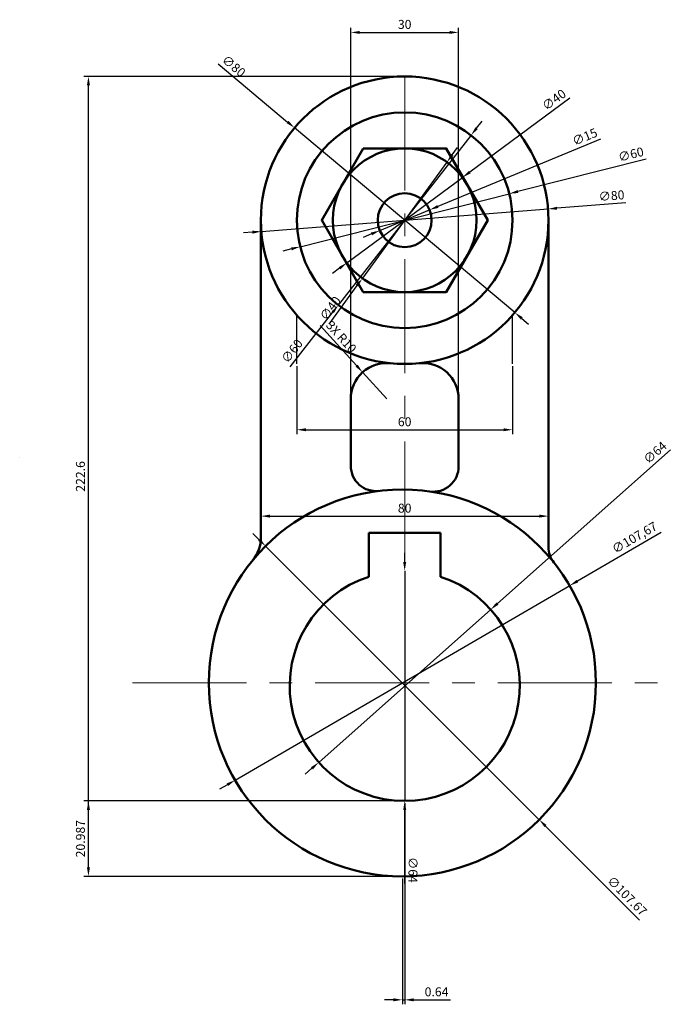
# Model space of a CAD drawing. Units: millimetres. Extents: x 3628 to 3809, y 2625 to 2899.
import ezdxf

# ---------------------------------------------------------------- set-up
doc = ezdxf.new("R2010")
doc.units = ezdxf.units.MM
doc.linetypes.add('CENTER', pattern=[50.8, 31.75, -6.35, 6.35, -6.35])
for name, color, linetype, lineweight in [('M-CNTR', 4, 'CENTER', 18), ('M-CONS', 8, 'Continuous', 13), ('M-DIMS', 2, 'Continuous', 25), ('M-OUTL', 7, 'Continuous', 50)]:
    doc.layers.add(name, color=color, linetype=linetype, lineweight=lineweight)
doc.styles.get("Standard").update_dxf_attribs({"font": 'arial.ttf'})
doc.dimstyles.new('ISO-25', dxfattribs={"dimtxt": 2.5, "dimasz": 2.5, "dimexe": 1.25, "dimexo": 0.625, "dimtad": 1, "dimtxsty": 'Standard', "dimcen": 2.5, "dimadec": 0, "dimazin": 0, "dimtfac": 1, "dimtmove": 0, "dimatfit": 3, "dimfxl": 1, "dimarcsym": 0})

# ---------------------------------------------------------------- blocks, each defined once
blk = doc.blocks.new('*D1')
at = {"layer": 'Defpoints', "color": 0, "transparency": 16777216}
for p in [(3758.59, 2734.73), (3710.75, 2692.22)]:
    blk.add_point(p, dxfattribs=at)
at = {"layer": 'M-DIMS', "color": 0, "lineweight": -2, "transparency": 16777216}
for p, q in [((3808.64, 2779.22), (3760.46, 2736.39)), ((3710.75, 2692.22), (3758.59, 2734.73)), ((3708.88, 2690.56), (3707.02, 2688.9))]:
    blk.add_line(p, q, dxfattribs=at)
at = {"layer": 'M-DIMS', "color": 0, "transparency": 16777216}
for points in [[(3760.18, 2736.71), (3760.74, 2736.08), (3758.59, 2734.73)], [(3708.61, 2690.87), (3709.16, 2690.25), (3710.75, 2692.22)]]:
    blk.add_solid(points, dxfattribs=at)
at = {"layer": 'M-DIMS', "color": 0, "transparency": 16777216, "insert": (3804.52, 2778.19), "char_height": 2.5, "attachment_point": 5, "rotation": 41.628}
blk.add_mtext('∅64', dxfattribs=at)
blk = doc.blocks.new('*D2')
at = {"layer": 'Defpoints', "color": 0, "transparency": 16777216}
for p in [(3750.76, 2854.98), (3718.59, 2831.21)]:
    blk.add_point(p, dxfattribs=at)
at = {"layer": 'M-DIMS', "color": 0, "lineweight": -2, "transparency": 16777216}
for p, q in [((3780.59, 2877.02), (3752.77, 2856.46)), ((3718.59, 2831.21), (3750.76, 2854.98)), ((3716.57, 2829.73), (3714.56, 2828.24))]:
    blk.add_line(p, q, dxfattribs=at)
at = {"layer": 'M-DIMS', "color": 0, "transparency": 16777216}
for points in [[(3752.52, 2856.8), (3753.02, 2856.13), (3750.76, 2854.98)], [(3716.33, 2830.06), (3716.82, 2829.39), (3718.59, 2831.21)]]:
    blk.add_solid(points, dxfattribs=at)
at = {"layer": 'M-DIMS', "color": 0, "transparency": 16777216, "insert": (3776.39, 2876.36), "char_height": 2.5, "attachment_point": 5, "rotation": 36.4548}
blk.add_mtext('∅40', dxfattribs=at)
blk = doc.blocks.new('*D3')
at = {"layer": 'Defpoints', "color": 0, "transparency": 16777216}
for p in [(3741.6, 2845.96), (3727.74, 2840.23)]:
    blk.add_point(p, dxfattribs=at)
at = {"layer": 'M-DIMS', "color": 0, "lineweight": -2, "transparency": 16777216}
for p, q in [((3789.15, 2865.64), (3743.91, 2846.92)), ((3727.74, 2840.23), (3741.6, 2845.96)), ((3725.43, 2839.27), (3723.12, 2838.32))]:
    blk.add_line(p, q, dxfattribs=at)
at = {"layer": 'M-DIMS', "color": 0, "transparency": 16777216}
for points in [[(3743.75, 2847.3), (3744.07, 2846.53), (3741.6, 2845.96)], [(3725.27, 2839.66), (3725.59, 2838.89), (3727.74, 2840.23)]]:
    blk.add_solid(points, dxfattribs=at)
at = {"layer": 'M-DIMS', "color": 0, "transparency": 16777216, "insert": (3784.89, 2866.01), "char_height": 2.5, "attachment_point": 5, "rotation": 22.4807}
blk.add_mtext('∅15', dxfattribs=at)
blk = doc.blocks.new('*D4')
at = {"layer": 'Defpoints', "color": 0, "transparency": 16777216}
for p in [(3763.75, 2850.46), (3705.59, 2835.73)]:
    blk.add_point(p, dxfattribs=at)
at = {"layer": 'M-DIMS', "color": 0, "lineweight": -2, "transparency": 16777216}
for p, q in [((3801.82, 2860.11), (3766.18, 2851.08)), ((3705.59, 2835.73), (3763.75, 2850.46)), ((3703.17, 2835.11), (3700.74, 2834.5))]:
    blk.add_line(p, q, dxfattribs=at)
at = {"layer": 'M-DIMS', "color": 0, "transparency": 16777216}
for points in [[(3766.07, 2851.48), (3766.28, 2850.67), (3763.75, 2850.46)], [(3703.07, 2835.52), (3703.27, 2834.71), (3705.59, 2835.73)]]:
    blk.add_solid(points, dxfattribs=at)
at = {"layer": 'M-DIMS', "color": 0, "transparency": 16777216, "insert": (3797.68, 2861.1), "char_height": 2.5, "attachment_point": 5, "rotation": 14.2196}
blk.add_mtext('∅60', dxfattribs=at)
blk = doc.blocks.new('*D5')
at = {"layer": 'Defpoints', "color": 0, "transparency": 16777216}
for p in [(3774.55, 2846.23), (3694.79, 2839.96)]:
    blk.add_point(p, dxfattribs=at)
at = {"layer": 'M-DIMS', "color": 0, "lineweight": -2, "transparency": 16777216}
for p, q in [((3796.15, 2847.93), (3777.04, 2846.43)), ((3694.79, 2839.96), (3774.55, 2846.23)), ((3692.3, 2839.76), (3689.81, 2839.57))]:
    blk.add_line(p, q, dxfattribs=at)
at = {"layer": 'M-DIMS', "color": 0, "transparency": 16777216}
for points in [[(3777.01, 2846.84), (3777.07, 2846.01), (3774.55, 2846.23)], [(3692.27, 2840.18), (3692.34, 2839.35), (3694.79, 2839.96)]]:
    blk.add_solid(points, dxfattribs=at)
at = {"layer": 'M-DIMS', "color": 0, "transparency": 16777216, "insert": (3792.23, 2849.6), "char_height": 2.5, "attachment_point": 5, "rotation": 4.4985}
blk.add_mtext('∅80', dxfattribs=at)
blk = doc.blocks.new('*D6')
at = {"layer": 'Defpoints', "color": 0, "transparency": 16777216}
for p in [(3704.67, 2803.1), (3764.67, 2803.1), (3764.67, 2784.78)]:
    blk.add_point(p, dxfattribs=at)
at = {"layer": 'M-DIMS', "color": 0, "lineweight": -2, "transparency": 16777216}
for p, q in [((3704.67, 2802.47), (3704.67, 2783.53)), ((3764.67, 2802.47), (3764.67, 2783.53)), ((3707.17, 2784.78), (3762.17, 2784.78))]:
    blk.add_line(p, q, dxfattribs=at)
at = {"layer": 'M-DIMS', "color": 0, "transparency": 16777216}
for points in [[(3707.17, 2785.2), (3707.17, 2784.36), (3704.67, 2784.78)], [(3762.17, 2785.2), (3762.17, 2784.36), (3764.67, 2784.78)]]:
    blk.add_solid(points, dxfattribs=at)
at = {"layer": 'M-DIMS', "color": 0, "transparency": 16777216, "insert": (3734.67, 2786.68), "char_height": 2.5, "attachment_point": 5}
blk.add_mtext('60', dxfattribs=at)
blk = doc.blocks.new('*D7')
at = {"layer": 'Defpoints', "color": 0, "transparency": 16777216}
for p in [(3780.57, 2741.39), (3687.5, 2687.25)]:
    blk.add_point(p, dxfattribs=at)
at = {"layer": 'M-DIMS', "color": 0, "lineweight": -2, "transparency": 16777216}
for p, q in [((3806.06, 2756.22), (3782.73, 2742.65)), ((3687.5, 2687.25), (3780.57, 2741.39)), ((3685.34, 2686), (3683.18, 2684.74))]:
    blk.add_line(p, q, dxfattribs=at)
at = {"layer": 'M-DIMS', "color": 0, "transparency": 16777216}
for points in [[(3782.52, 2743.01), (3782.94, 2742.29), (3780.57, 2741.39)], [(3685.13, 2686.36), (3685.55, 2685.64), (3687.5, 2687.25)]]:
    blk.add_solid(points, dxfattribs=at)
at = {"layer": 'M-DIMS', "color": 0, "transparency": 16777216, "insert": (3798.76, 2754.49), "char_height": 2.5, "attachment_point": 5, "rotation": 30.1871}
blk.add_mtext('∅107,67', dxfattribs=at)
blk = doc.blocks.new('*D8')
at = {"layer": 'Defpoints', "color": 0, "transparency": 16777216}
for p in [(3774.67, 2760.74), (3694.67, 2754.8), (3774.67, 2754.8)]:
    blk.add_point(p, dxfattribs=at)
at = {"layer": 'M-DIMS', "color": 0, "lineweight": -2, "transparency": 16777216}
for p, q in [((3694.67, 2755.42), (3694.67, 2761.99)), ((3697.17, 2760.74), (3772.17, 2760.74)), ((3774.67, 2755.42), (3774.67, 2761.99))]:
    blk.add_line(p, q, dxfattribs=at)
at = {"layer": 'M-DIMS', "color": 0, "transparency": 16777216}
for points in [[(3697.17, 2761.16), (3697.17, 2760.33), (3694.67, 2760.74)], [(3772.17, 2761.16), (3772.17, 2760.33), (3774.67, 2760.74)]]:
    blk.add_solid(points, dxfattribs=at)
at = {"layer": 'M-DIMS', "color": 0, "transparency": 16777216, "insert": (3734.67, 2762.64), "char_height": 2.5, "attachment_point": 5}
blk.add_mtext('80', dxfattribs=at)
blk = doc.blocks.new('*D9')
at = {"layer": 'Defpoints', "color": 0, "transparency": 16777216}
for p in [(3646.69, 2681.48), (3734.67, 2681.48), (3734.03, 2660.49)]:
    blk.add_point(p, dxfattribs=at)
at = {"layer": 'M-DIMS', "color": 0, "lineweight": -2, "transparency": 16777216}
for p, q in [((3734.05, 2681.48), (3645.44, 2681.48)), ((3646.69, 2662.99), (3646.69, 2678.98)), ((3733.41, 2660.49), (3645.44, 2660.49))]:
    blk.add_line(p, q, dxfattribs=at)
at = {"layer": 'M-DIMS', "color": 0, "transparency": 16777216}
for points in [[(3646.27, 2678.98), (3647.11, 2678.98), (3646.69, 2681.48)], [(3646.27, 2662.99), (3647.11, 2662.99), (3646.69, 2660.49)]]:
    blk.add_solid(points, dxfattribs=at)
at = {"layer": 'M-DIMS', "color": 0, "transparency": 16777216, "insert": (3644.79, 2670.98), "char_height": 2.5, "attachment_point": 5, "rotation": 90}
blk.add_mtext('20.987', dxfattribs=at)
blk = doc.blocks.new('*D10')
at = {"layer": 'Defpoints', "color": 0, "transparency": 16777216}
for p in [(3749.67, 2895.36), (3719.67, 2793.35), (3749.67, 2793.35)]:
    blk.add_point(p, dxfattribs=at)
at = {"layer": 'M-DIMS', "color": 0, "lineweight": -2, "transparency": 16777216}
for p, q in [((3719.67, 2793.97), (3719.67, 2896.61)), ((3749.67, 2793.97), (3749.67, 2896.61)), ((3722.17, 2895.36), (3747.17, 2895.36))]:
    blk.add_line(p, q, dxfattribs=at)
at = {"layer": 'M-DIMS', "color": 0, "transparency": 16777216}
for points in [[(3722.17, 2895.77), (3722.17, 2894.94), (3719.67, 2895.36)], [(3747.17, 2895.77), (3747.17, 2894.94), (3749.67, 2895.36)]]:
    blk.add_solid(points, dxfattribs=at)
at = {"layer": 'M-DIMS', "color": 0, "transparency": 16777216, "insert": (3734.67, 2897.26), "char_height": 2.5, "attachment_point": 5}
blk.add_mtext('30', dxfattribs=at)
blk = doc.blocks.new('*D11')
at = {"layer": 'Defpoints', "color": 0, "transparency": 16777216}
for p in [(3646.69, 2883.1), (3734.67, 2883.1), (3734.03, 2660.49)]:
    blk.add_point(p, dxfattribs=at)
at = {"layer": 'M-DIMS', "color": 0, "lineweight": -2, "transparency": 16777216}
for p, q in [((3734.05, 2883.1), (3645.44, 2883.1)), ((3646.69, 2662.99), (3646.69, 2880.6)), ((3733.41, 2660.49), (3645.44, 2660.49))]:
    blk.add_line(p, q, dxfattribs=at)
at = {"layer": 'M-DIMS', "color": 0, "transparency": 16777216}
for points in [[(3646.27, 2880.6), (3647.11, 2880.6), (3646.69, 2883.1)], [(3646.27, 2662.99), (3647.11, 2662.99), (3646.69, 2660.49)]]:
    blk.add_solid(points, dxfattribs=at)
at = {"layer": 'M-DIMS', "color": 0, "transparency": 16777216, "insert": (3644.79, 2771.79), "char_height": 2.5, "attachment_point": 5, "rotation": 90}
blk.add_mtext('222.6', dxfattribs=at)
blk = doc.blocks.new('*D12')
at = {"layer": 'Defpoints', "color": 0, "transparency": 16777216}
for p in [(3734.67, 2681.48), (3734.03, 2660.49), (3734.67, 2626.13)]:
    blk.add_point(p, dxfattribs=at)
at = {"layer": 'M-DIMS', "color": 0, "lineweight": -2, "transparency": 16777216}
for p, q in [((3734.67, 2680.85), (3734.67, 2624.88)), ((3734.03, 2659.86), (3734.03, 2624.88)), ((3731.53, 2626.13), (3729.03, 2626.13)), ((3734.03, 2626.13), (3734.67, 2626.13)), ((3737.17, 2626.13), (3747.41, 2626.13))]:
    blk.add_line(p, q, dxfattribs=at)
at = {"layer": 'M-DIMS', "color": 0, "transparency": 16777216}
for points in [[(3731.53, 2626.55), (3731.53, 2625.71), (3734.03, 2626.13)], [(3737.17, 2626.55), (3737.17, 2625.71), (3734.67, 2626.13)]]:
    blk.add_solid(points, dxfattribs=at)
at = {"layer": 'M-DIMS', "color": 0, "transparency": 16777216, "insert": (3743.54, 2628.03), "char_height": 2.5, "attachment_point": 5}
blk.add_mtext('0.64', dxfattribs=at)
blk = doc.blocks.new('*D13')
at = {"layer": 'Defpoints', "color": 0, "transparency": 16777216}
for p in [(3695.97, 2752.39), (3772.1, 2676.25)]:
    blk.add_point(p, dxfattribs=at)
at = {"layer": 'M-DIMS', "color": 0, "lineweight": -2, "transparency": 16777216}
for p, q in [((3694.2, 2754.16), (3692.43, 2755.93)), ((3695.97, 2752.39), (3772.1, 2676.25)), ((3800.01, 2648.34), (3773.86, 2674.49))]:
    blk.add_line(p, q, dxfattribs=at)
at = {"layer": 'M-DIMS', "color": 0, "transparency": 16777216}
for points in [[(3694.5, 2754.46), (3693.91, 2753.87), (3695.97, 2752.39)], [(3774.16, 2674.78), (3773.57, 2674.19), (3772.1, 2676.25)]]:
    blk.add_solid(points, dxfattribs=at)
at = {"layer": 'M-DIMS', "color": 0, "transparency": 16777216, "insert": (3796.33, 2654.81), "char_height": 2.5, "attachment_point": 5, "rotation": 314.9952}
blk.add_mtext('∅107.67', dxfattribs=at)
blk = doc.blocks.new('*D14')
at = {"layer": 'Defpoints', "color": 0, "transparency": 16777216}
for p in [(3704.03, 2868.8), (3765.32, 2817.39)]:
    blk.add_point(p, dxfattribs=at)
at = {"layer": 'M-DIMS', "color": 0, "lineweight": -2, "transparency": 16777216}
for p, q in [((3682.75, 2886.65), (3702.11, 2870.41)), ((3765.32, 2817.39), (3704.03, 2868.8)), ((3767.23, 2815.78), (3769.15, 2814.17))]:
    blk.add_line(p, q, dxfattribs=at)
at = {"layer": 'M-DIMS', "color": 0, "transparency": 16777216}
for points in [[(3702.38, 2870.73), (3701.84, 2870.09), (3704.03, 2868.8)], [(3767.5, 2816.1), (3766.96, 2815.46), (3765.32, 2817.39)]]:
    blk.add_solid(points, dxfattribs=at)
at = {"layer": 'M-DIMS', "color": 0, "transparency": 16777216, "insert": (3686.91, 2885.74), "char_height": 2.5, "attachment_point": 5, "rotation": 320.0072}
blk.add_mtext('∅80', dxfattribs=at)
blk = doc.blocks.new('*D15')
at = {"layer": 'Defpoints', "color": 0, "transparency": 16777216}
for p in [(3753.14, 2866.74), (3716.2, 2819.45)]:
    blk.add_point(p, dxfattribs=at)
at = {"layer": 'M-DIMS', "color": 0, "lineweight": -2, "transparency": 16777216}
for p, q in [((3754.68, 2868.71), (3756.22, 2870.68)), ((3753.14, 2866.74), (3716.2, 2819.45)), ((3702.8, 2802.3), (3714.66, 2817.48))]:
    blk.add_line(p, q, dxfattribs=at)
at = {"layer": 'M-DIMS', "color": 0, "transparency": 16777216}
for points in [[(3754.35, 2868.96), (3755.01, 2868.45), (3753.14, 2866.74)], [(3714.34, 2817.74), (3714.99, 2817.23), (3716.2, 2819.45)]]:
    blk.add_solid(points, dxfattribs=at)
at = {"layer": 'M-DIMS', "color": 0, "transparency": 16777216, "insert": (3703.57, 2806.48), "char_height": 2.5, "attachment_point": 5, "rotation": 52.0029}
blk.add_mtext('∅60', dxfattribs=at)
blk = doc.blocks.new('*D16')
at = {"layer": 'Defpoints', "color": 0, "transparency": 16777216}
for p in [(3746.44, 2859.27), (3722.9, 2826.92)]:
    blk.add_point(p, dxfattribs=at)
at = {"layer": 'M-DIMS', "color": 0, "lineweight": -2, "transparency": 16777216}
for p, q in [((3747.91, 2861.29), (3749.38, 2863.31)), ((3746.44, 2859.27), (3722.9, 2826.92)), ((3713.62, 2814.17), (3721.43, 2824.9))]:
    blk.add_line(p, q, dxfattribs=at)
at = {"layer": 'M-DIMS', "color": 0, "transparency": 16777216}
for points in [[(3747.57, 2861.53), (3748.25, 2861.04), (3746.44, 2859.27)], [(3721.1, 2825.15), (3721.77, 2824.66), (3722.9, 2826.92)]]:
    blk.add_solid(points, dxfattribs=at)
at = {"layer": 'M-DIMS', "color": 0, "transparency": 16777216, "insert": (3714.25, 2818.38), "char_height": 2.5, "attachment_point": 5, "rotation": 53.9542}
blk.add_mtext('∅40', dxfattribs=at)
blk = doc.blocks.new('*D17')
at = {"layer": 'Defpoints', "color": 0, "transparency": 16777216}
for p in [(3734.67, 2745.48), (3734.67, 2681.48)]:
    blk.add_point(p, dxfattribs=at)
at = {"layer": 'M-DIMS', "color": 0, "lineweight": -2, "transparency": 16777216}
for p, q in [((3734.67, 2747.98), (3734.67, 2750.48)), ((3734.67, 2745.48), (3734.67, 2681.48)), ((3734.67, 2658.51), (3734.67, 2678.98))]:
    blk.add_line(p, q, dxfattribs=at)
at = {"layer": 'M-DIMS', "color": 0, "transparency": 16777216}
for points in [[(3735.09, 2747.98), (3734.25, 2747.98), (3734.67, 2745.48)], [(3735.09, 2678.98), (3734.26, 2678.98), (3734.67, 2681.48)]]:
    blk.add_solid(points, dxfattribs=at)
at = {"layer": 'M-DIMS', "color": 0, "transparency": 16777216, "insert": (3736.64, 2662.28), "char_height": 2.5, "attachment_point": 5, "rotation": 270.0006}
blk.add_mtext('∅64', dxfattribs=at)
blk = doc.blocks.new('*D18')
at = {"layer": 'Defpoints', "color": 0, "transparency": 16777216}
for p in [(3722.96, 2800.76), (3729.67, 2793.35)]:
    blk.add_point(p, dxfattribs=at)
at = {"layer": 'M-DIMS', "color": 0, "lineweight": -2, "transparency": 16777216}
for p, q in [((3711.17, 2813.8), (3721.29, 2802.62)), ((3729.67, 2793.35), (3722.96, 2800.76))]:
    blk.add_line(p, q, dxfattribs=at)
at = {"layer": 'M-DIMS', "color": 0, "transparency": 16777216}
blk.add_solid([(3721.6, 2802.9), (3720.98, 2802.34), (3722.96, 2800.76)], dxfattribs=at)
at = {"layer": 'M-DIMS', "color": 0, "transparency": 16777216, "insert": (3716.8, 2810.41), "char_height": 2.5, "attachment_point": 5, "rotation": 312.1323}
blk.add_mtext('3X R10', dxfattribs=at)

msp = doc.modelspace()

# ---------------------------------------------------------------- linework, layer by layer
at = {"layer": 'M-CNTR'}
for p, q in [((3734.6717, 2883.0951), (3734.6717, 2638.3904)), ((3658.9492, 2714.3233), (3809.1168, 2714.3233))]:
    msp.add_line(p, q, dxfattribs=at)
at = {"layer": 'M-CONS'}
for p, q in [((3774.6717, 2821.5551), (3774.6717, 2821.5551)), ((3774.6717, 2821.5551), (3774.6717, 2821.5551)), ((3627.5689, 2777.1809), (3627.5689, 2777.1809)), ((3627.5689, 2777.1809), (3627.5689, 2777.1809)), ((3766.6717, 2713.4763), (3766.8495, 2713.4763))]:
    msp.add_line(p, q, dxfattribs=at)
at = {"layer": 'M-DIMS'}
for p, q in [((3704.6717, 2803.0951), (3704.6717, 2816.6376)), ((3764.6717, 2803.0951), (3764.6717, 2816.6376))]:
    msp.add_line(p, q, dxfattribs=at)
at = {"layer": 'M-OUTL'}
for p, q in [((3694.6717, 2843.0951), (3694.6717, 2782.7837)), ((3774.6717, 2843.0951), (3774.6717, 2792.4695)), ((3719.6717, 2793.3457), (3719.6717, 2774.7105)), ((3749.6717, 2793.3457), (3749.6717, 2774.541)), ((3774.6717, 2781.856), (3774.6717, 2792.4695)), ((3694.6717, 2782.7837), (3694.6717, 2754.7988)), ((3774.6717, 2781.856), (3774.6717, 2752.1566)), ((3724.6717, 2756.1035), (3744.6717, 2756.1035)), ((3724.6717, 2756.1035), (3724.6717, 2743.8736)), ((3744.6717, 2756.1035), (3744.6717, 2743.8736)), ((3744.6717, 2756.1035), (3744.6717, 2743.8736)), ((3744.6717, 2756.1035), (3744.6717, 2743.8736))]:
    msp.add_line(p, q, dxfattribs=at)
msp.add_lwpolyline([(3723.1247, 2863.0951), (3711.5777, 2843.0951), (3723.1247, 2823.0951), (3746.2187, 2823.0951), (3757.7657, 2843.0951), (3746.2187, 2863.0951)], close=True, dxfattribs=at)
for centre, radius in [((3734.6717, 2843.0951), 40), ((3734.6717, 2843.0951), 30), ((3734.6717, 2843.0951), 30), ((3734.6717, 2843.0951), 20), ((3734.6717, 2843.0951), 7.5), ((3734.033, 2714.3233), 53.8342)]:
    msp.add_circle(centre, radius, dxfattribs=at)
for centre, radius, start, end in [((3729.6717, 2793.3457), 10, 84.26083, 180), ((3739.6717, 2793.3457), 10, 0, 95.73917), ((3726.6717, 2774.7105), 7, 180, 276.950187), ((3742.6717, 2774.541), 7, 261.836205, 0), ((3684.6717, 2754.7988), 10, 320.648784, 0), ((3781.6717, 2752.1566), 7, 180, 218.455632), ((3734.6717, 2713.4763), 32, 108.209957, 71.790043)]:
    msp.add_arc(centre, radius, start, end, dxfattribs=at)

# ---------------------------------------------------------------- dimensions: what is measured, and where the dimension line sits
at = {"layer": 'M-DIMS'}
for base, p1, p2, override, picture, middle in [((3749.6717, 2895.3551), (3719.6717, 2793.3457), (3749.6717, 2793.3457), {"dimdec": 0, "dimlfac": 1, "dimrnd": 0, "dimzin": 0, "dimdsep": 46, "dimlunit": 2}, '*D10', (3734.6717, 2897.2574)), ((3764.6717, 2784.7789), (3704.6717, 2803.0951), (3764.6717, 2803.0951), {"dimclrd": 0, "dimclre": 0, "dimclrt": 0}, '*D6', (3734.6717, 2786.6803)), ((3774.6717, 2760.7428), (3694.6717, 2754.7988), (3774.6717, 2754.7988), {"dimclrd": 0, "dimclre": 0, "dimclrt": 0}, '*D8', (3734.6717, 2762.6442)), ((3734.6717, 2626.1304), (3734.033, 2660.4891), (3734.6717, 2681.4763), {"dimdec": 2, "dimlfac": 1, "dimrnd": 0, "dimzin": 0, "dimdsep": 46, "dimlunit": 2}, '*D12', (3743.5385, 2628.0318))]:
    dim = msp.add_linear_dim(base=base, p1=p1, p2=p2, dimstyle='ISO-25', override=override, dxfattribs=at)
    dim.commit()
    dim.dimension.update_dxf_attribs({"geometry": picture, "text_midpoint": middle})
for p1, p2, override, picture, middle in [((3765.3167, 2817.3875), (3704.0267, 2868.8028), {"dimdec": 0, "dimlfac": 1, "dimrnd": 0, "dimzin": 0, "dimdsep": 46, "dimlunit": 2}, '*D14', (3685.6397, 2884.2274)), ((3718.5852, 2831.2113), (3750.7582, 2854.9789), {"dimclrd": 0, "dimclre": 0, "dimclrt": 0}, '*D2', (3777.5577, 2874.7768)), ((3753.1404, 2866.7364), (3716.203, 2819.4539), {"dimdec": 0, "dimlfac": 1, "dimrnd": 0, "dimzin": 0, "dimdsep": 46, "dimlunit": 2}, '*D15', (3705.1218, 2805.2691)), ((3727.7416, 2840.2273), (3741.6018, 2845.9629), {"dimclrd": 0, "dimclre": 0, "dimclrt": 0}, '*D3', (3785.6478, 2864.19)), ((3705.5908, 2835.726), (3763.7525, 2850.4643), {"dimclrd": 0, "dimclre": 0, "dimclrt": 0}, '*D4', (3798.1682, 2859.1853)), ((3746.4403, 2859.266), (3722.903, 2826.9242), {"dimdec": 0, "dimlfac": 1, "dimrnd": 0, "dimzin": 0, "dimdsep": 46, "dimlunit": 2}, '*D16', (3715.8419, 2817.2216)), ((3694.7949, 2839.9578), (3774.5485, 2846.2324), {"dimclrd": 0, "dimclre": 0, "dimclrt": 0}, '*D5', (3792.3896, 2847.6361)), ((3710.7525, 2692.2189), (3758.5908, 2734.7336), {"dimclrd": 0, "dimclre": 0, "dimclrt": 0}, '*D1', (3805.826, 2776.7122)), ((3687.4994, 2687.2541), (3780.5667, 2741.3925), {"dimclrd": 0, "dimclre": 0, "dimclrt": 0}, '*D7', (3799.8547, 2752.6125)), ((3695.9696, 2752.393), (3772.0964, 2676.2536), {"dimdec": 2, "dimlfac": 1, "dimrnd": 0, "dimzin": 0, "dimdsep": 46, "dimlunit": 2}, '*D13', (3794.9344, 2653.4118)), ((3734.6714, 2745.4763), (3734.672, 2681.4763), {"dimdec": 0, "dimlfac": 1, "dimrnd": 0, "dimzin": 0, "dimdsep": 46, "dimlunit": 2}, '*D17', (3734.6722, 2662.2763))]:
    dim = msp.add_diameter_dim_2p(p1=p1, p2=p2, dimstyle='ISO-25', override=override, dxfattribs=at)
    dim.commit()
    dim.dimension.update_dxf_attribs({"geometry": picture, "text_midpoint": middle, "dimtype": 163})
for base, p2, override, picture, middle in [((3646.6892, 2883.0951), (3734.6717, 2883.0951), {"dimdec": 1, "dimlfac": 1, "dimrnd": 0, "dimzin": 0, "dimdsep": 46, "dimlunit": 2}, '*D11', (3644.7878, 2771.7921)), ((3646.6892, 2681.4763), (3734.6717, 2681.4763), {"dimdec": 3, "dimlfac": 1, "dimrnd": 0, "dimzin": 0, "dimdsep": 46, "dimlunit": 2}, '*D9', (3644.7878, 2670.9827))]:
    dim = msp.add_linear_dim(base=base, p1=(3734.033, 2660.4891), p2=p2, angle=90, dimstyle='ISO-25', override=override, dxfattribs=at)
    dim.commit()
    dim.dimension.update_dxf_attribs({"geometry": picture, "text_midpoint": middle})
dim = msp.add_radius_dim(center=(3729.6717, 2793.3457), mpoint=(3722.9632, 2800.7617), text='3X <>', dimstyle='ISO-25', override={"dimdec": 0, "dimlfac": 1, "dimrnd": 0, "dimzin": 0, "dimdsep": 46, "dimlunit": 2}, dxfattribs=at)
dim.commit()
dim.dimension.update_dxf_attribs({"geometry": '*D18', "text_midpoint": (3716.7984, 2810.4125)})

doc.saveas('drawing.dxf')
